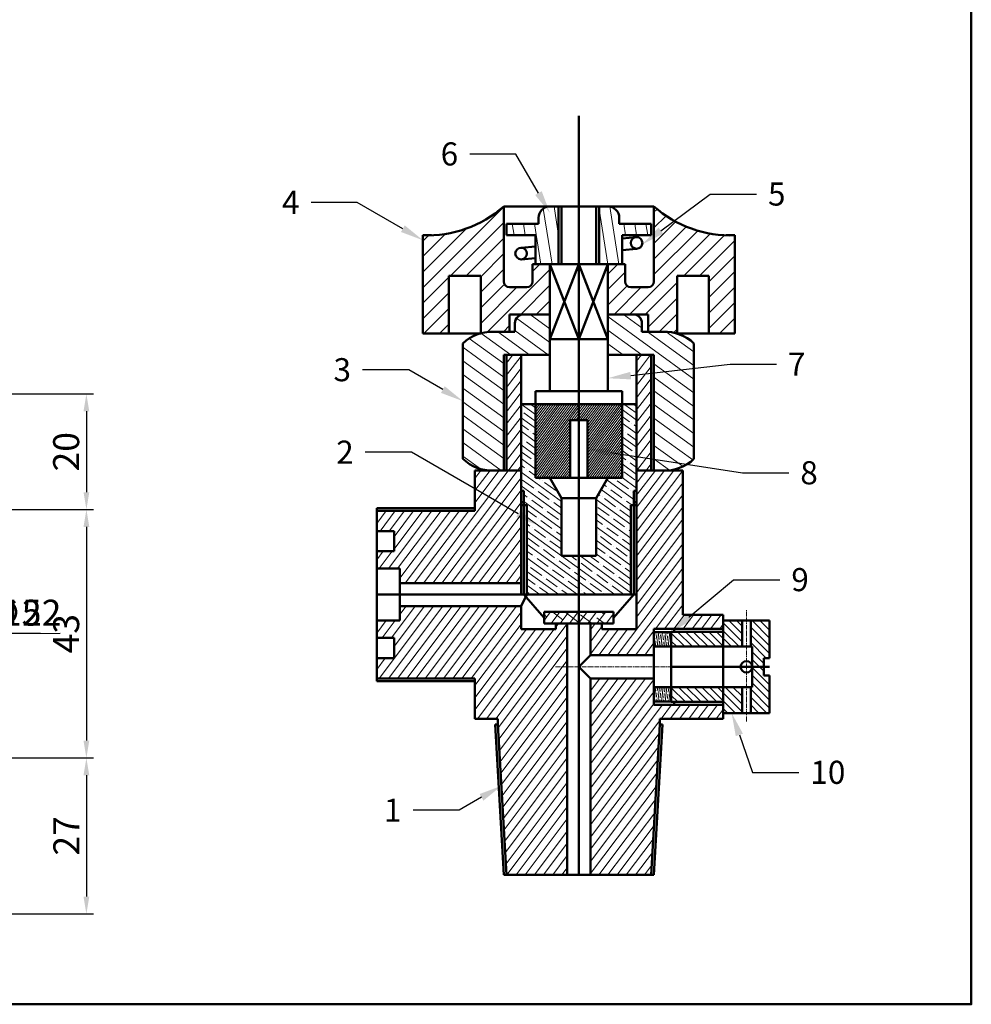
# Model space of a CAD drawing. Units: millimetres. Extents: x 418 to 773, y -46 to 294.
# Tile 6 of 7: x 609 to 773, y -46 to 124. Entities that reach past the tile are written whole.
import ezdxf
from ezdxf import colors
from ezdxf.entities.mleader import LeaderData, LeaderLine
from ezdxf.math import Vec2, Vec3

# ---------------------------------------------------------------- set-up
doc = ezdxf.new("R2010")
doc.units = ezdxf.units.MM
doc.header["$LTSCALE"] = 0.2
doc.linetypes.add('CENTER2', pattern=[28.575, 19.05, -3.175, 3.175, -3.175])
for name, color, linetype, lineweight in [('M-CNTR', 1, 'CENTER2', 18), ('M-DIMS', 2, 'Continuous', 25), ('M-HATC', 8, 'Continuous', 18), ('M-OUTL', 7, 'Continuous', 50), ('M-TEXT', 3, 'Continuous', 25), ('M-TTLB', 7, 'Continuous', 50)]:
    doc.layers.add(name, color=color, linetype=linetype, lineweight=lineweight)
doc.styles.get("Standard").update_dxf_attribs({"font": 'arial.ttf'})
doc.dimstyles.new('ISO-25', dxfattribs={"dimtxt": 4.5, "dimasz": 3, "dimexe": 1.25, "dimexo": 0.625, "dimtad": 1, "dimdec": 1, "dimtxsty": 'Standard', "dimcen": 2.5, "dimadec": 0, "dimazin": 0, "dimtfac": 1, "dimtdec": 1, "dimtmove": 0, "dimatfit": 3, "dimfxl": 1, "dimarcsym": 0})

# ---------------------------------------------------------------- blocks, each defined once
blk = doc.blocks.new('*D90')
at = {"layer": 'Defpoints', "color": 0, "ltscale": 0.2, "transparency": 16777216}
for p in [(600.02, 59.18), (601.02, 39.18), (620.1, 39.18)]:
    blk.add_point(p, dxfattribs=at)
at = {"layer": 'M-DIMS', "color": 0, "lineweight": -2, "ltscale": 0.2, "transparency": 16777216}
for p, q in [((600.64, 59.18), (621.35, 59.18)), ((620.1, 56.18), (620.1, 42.18)), ((601.64, 39.18), (621.35, 39.18))]:
    blk.add_line(p, q, dxfattribs=at)
at = {"layer": 'M-DIMS', "color": 0, "ltscale": 0.2, "transparency": 16777216}
for points in [[(619.6, 56.18), (620.6, 56.18), (620.1, 59.18)], [(619.6, 42.18), (620.6, 42.18), (620.1, 39.18)]]:
    blk.add_solid(points, dxfattribs=at)
at = {"layer": 'M-DIMS', "color": 0, "ltscale": 0.2, "transparency": 16777216, "insert": (617.18, 49.18), "char_height": 4.5, "attachment_point": 5, "rotation": 90}
blk.add_mtext('20', dxfattribs=at)
blk = doc.blocks.new('*D91')
at = {"layer": 'Defpoints', "color": 0, "ltscale": 0.2, "transparency": 16777216}
for p in [(611.5, 39.18), (604.02, -3.82), (620.1, -3.82)]:
    blk.add_point(p, dxfattribs=at)
at = {"layer": 'M-DIMS', "color": 0, "lineweight": -2, "ltscale": 0.2, "transparency": 16777216}
for p, q in [((612.12, 39.18), (621.35, 39.18)), ((620.1, 36.18), (620.1, -0.82)), ((604.64, -3.82), (621.35, -3.82))]:
    blk.add_line(p, q, dxfattribs=at)
at = {"layer": 'M-DIMS', "color": 0, "ltscale": 0.2, "transparency": 16777216}
for points in [[(619.6, 36.18), (620.6, 36.18), (620.1, 39.18)], [(619.6, -0.82), (620.6, -0.82), (620.1, -3.82)]]:
    blk.add_solid(points, dxfattribs=at)
at = {"layer": 'M-DIMS', "color": 0, "ltscale": 0.2, "transparency": 16777216, "insert": (617.18, 17.68), "char_height": 4.5, "attachment_point": 5, "rotation": 90}
blk.add_mtext('43', dxfattribs=at)
blk = doc.blocks.new('*D92')
at = {"layer": 'Defpoints', "color": 0, "ltscale": 0.2, "transparency": 16777216}
for p in [(608.93, -3.82), (592.52, -30.82), (620.1, -30.82)]:
    blk.add_point(p, dxfattribs=at)
at = {"layer": 'M-DIMS', "color": 0, "lineweight": -2, "ltscale": 0.2, "transparency": 16777216}
for p, q in [((609.56, -3.82), (621.35, -3.82)), ((620.1, -6.82), (620.1, -27.82)), ((593.14, -30.82), (621.35, -30.82))]:
    blk.add_line(p, q, dxfattribs=at)
at = {"layer": 'M-DIMS', "color": 0, "ltscale": 0.2, "transparency": 16777216}
for points in [[(619.6, -6.82), (620.6, -6.82), (620.1, -3.82)], [(619.6, -27.82), (620.6, -27.82), (620.1, -30.82)]]:
    blk.add_solid(points, dxfattribs=at)
at = {"layer": 'M-DIMS', "color": 0, "ltscale": 0.2, "transparency": 16777216, "insert": (617.22, -17.32), "char_height": 4.5, "attachment_point": 5, "rotation": 90}
blk.add_mtext('27', dxfattribs=at)
blk = doc.blocks.new('*D102')
at = {"layer": 'Defpoints', "color": 0, "ltscale": 0.2, "transparency": 16777216}
for p in [(575.02, 17.68), (597.02, 17.68)]:
    blk.add_point(p, dxfattribs=at)
at = {"layer": 'M-DIMS', "color": 0, "lineweight": -2, "ltscale": 0.2, "transparency": 16777216}
for p, q in [((572.02, 17.68), (569.02, 17.68)), ((575.02, 17.68), (597.02, 17.68)), ((615.56, 17.69), (600.02, 17.68))]:
    blk.add_line(p, q, dxfattribs=at)
at = {"layer": 'M-DIMS', "color": 0, "ltscale": 0.2, "transparency": 16777216}
for points in [[(572.02, 18.18), (572.02, 17.18), (575.02, 17.68)], [(600.02, 18.19), (600.02, 17.19), (597.02, 17.68)]]:
    blk.add_solid(points, dxfattribs=at)
at = {"layer": 'M-DIMS', "color": 0, "ltscale": 0.2, "transparency": 16777216, "insert": (609.29, 20.73), "char_height": 4.5, "attachment_point": 5, "rotation": 0.0004}
blk.add_mtext('∅22', dxfattribs=at)
blk = doc.blocks.new('*D103')
at = {"layer": 'Defpoints', "color": 0, "ltscale": 0.2, "transparency": 16777216}
for p in [(578.52, 17.68), (593.52, 17.69)]:
    blk.add_point(p, dxfattribs=at)
at = {"layer": 'M-DIMS', "color": 0, "lineweight": -2, "ltscale": 0.2, "transparency": 16777216}
for p, q in [((575.52, 17.68), (572.52, 17.68)), ((578.52, 17.68), (593.52, 17.69)), ((612.14, 17.69), (596.52, 17.69))]:
    blk.add_line(p, q, dxfattribs=at)
at = {"layer": 'M-DIMS', "color": 0, "ltscale": 0.2, "transparency": 16777216}
for points in [[(575.52, 18.18), (575.52, 17.18), (578.52, 17.68)], [(596.52, 18.19), (596.52, 17.19), (593.52, 17.69)]]:
    blk.add_solid(points, dxfattribs=at)
at = {"layer": 'M-DIMS', "color": 0, "ltscale": 0.2, "transparency": 16777216, "insert": (605.83, 20.73), "char_height": 4.5, "attachment_point": 5, "rotation": 0.0006}
blk.add_mtext('∅15', dxfattribs=at)

msp = doc.modelspace()

# ---------------------------------------------------------------- hatches: boundary and pattern name
at = {"layer": 'M-HATC', "ltscale": 0.2}
h = msp.add_hatch(dxfattribs=at)
h.set_pattern_fill('ANSI31', color=256, scale=0.6)
h.paths.add_polyline_path([(732.3444, 86.646, -0.1927282), (718.3444, 91.646), (718.3444, 78.646, -0.41421356), (717.3444, 77.646), (714.3444, 77.646, -0.41421356), (713.3444, 78.646), (713.3444, 81.646), (710.3444, 81.646), (710.3444, 72.9399), (717.3444, 72.9399), (717.3444, 69.9399), (719.8686, 69.9399, -0.08679952), (722.3398, 69.646), (722.3444, 69.646), (722.3444, 79.646), (727.8444, 79.646), (727.8444, 69.646), (732.3444, 69.646)])
h.paths.add_polyline_path([(692.3444, 91.646, -0.1927282), (678.3444, 86.646), (678.3444, 69.646), (682.8444, 69.646), (682.8444, 79.646), (688.3444, 79.646), (688.3444, 69.6846, -0.07535531), (690.4992, 69.9399), (693.3444, 69.9399), (693.3444, 72.9399), (700.3444, 72.9399), (700.3444, 81.646), (697.3444, 81.646), (697.3444, 78.646, -0.41421356), (696.3444, 77.646), (693.3444, 77.646, -0.41421356), (692.3444, 78.646)])
h = msp.add_hatch(dxfattribs=at)
h.set_pattern_fill('ANSI31', color=256, scale=0.6, angle=54)
h.paths.add_polyline_path([(712.8444, 86.646), (717.8444, 86.646), (717.8444, 88.646), (712.3444, 88.646), (712.3444, 89.646, 0.41421356), (710.3444, 91.646), (708.8444, 91.646), (708.8444, 81.646), (712.8444, 81.646)])
h.paths.add_polyline_path([(701.8444, 91.646), (700.3444, 91.646, 0.41421356), (698.3444, 89.646), (698.3444, 88.646), (692.8444, 88.646), (692.8444, 86.646), (697.8444, 86.646), (697.8444, 81.646), (701.8444, 81.646)])
h = msp.add_hatch(dxfattribs=at)
h.set_pattern_fill('ANSI31', color=256, scale=0.6, angle=99)
h.paths.add_polyline_path([(692.3444, 65.9399), (695.3444, 65.9399), (700.3444, 65.9399), (700.3444, 68.646), (700.3444, 72.9399), (695.7641, 72.9399, 0.41421356), (694.2641, 71.4399), (694.2641, 69.9399), (690.029, 69.9399, 0.05904189), (688.3444, 69.6846), (688.3444, 69.646), (688.2094, 69.646, 0.11920158), (685.2641, 67.9399), (685.2641, 47.9399, 0.18451463), (690.029, 45.9399), (692.3444, 45.9399)])
h.paths.add_polyline_path([(725.2641, 67.9399, 0.17937471), (720.6597, 69.9399), (716.2641, 69.9399), (716.2641, 71.4399, 0.41421356), (714.7641, 72.9399), (710.3444, 72.9399), (710.3444, 72.646), (710.3444, 68.646), (710.3444, 65.9399), (715.3444, 65.9399), (718.3444, 65.9399), (718.3444, 45.9399), (720.6597, 45.9399, 0.17937471), (725.2641, 47.9399)])
h = msp.add_hatch(dxfattribs=at)
h.set_pattern_fill('ANSI31', color=256, scale=0.4, angle=8)
h.set_pattern_definition([(53, (-256.1481, -162.8936), (-1.0142671, 0.764305), [])])
h.paths.add_polyline_path([(707.3444, -24.0601), (717.8435, -24.0601), (719.3452, 1.9687), (719.3452, 2.9399), (730.3444, 2.9399), (730.3444, 5.3599), (718.3444, 5.3599), (718.3444, 9.9399), (707.3444, 9.9399)])
h.paths.add_polyline_path([(718.3444, 18.5199), (730.3444, 18.5199), (730.3444, 20.9399), (723.3444, 20.9399), (723.3444, 45.9399), (717.8444, 45.9399), (717.8444, 65.9399), (715.3444, 65.9399), (715.3444, 39.9399), (715.3444, 24.4399), (715.3444, 18.4399), (709.3444, 18.4399), (709.3444, 19.4399), (707.3444, 19.4399), (707.3444, 13.9399), (718.3444, 13.9399)])
h.paths.add_polyline_path([(695.3444, 39.9399), (695.3444, 65.9399), (692.8444, 65.9399), (692.8444, 45.9399), (687.3444, 45.9399), (687.3444, 38.9399), (670.3444, 38.9399), (670.3444, 35.4399), (673.3444, 35.4399), (673.3444, 31.9399), (670.3444, 31.9399), (670.3444, 28.9399), (674.3444, 28.9399), (674.3444, 26.4399), (695.3444, 26.4399)])
h.paths.add_polyline_path([(687.3444, 9.9399), (687.3444, 2.9399), (691.3444, 2.9399), (691.3444, 1.9543), (692.8452, -24.0601), (703.3444, -24.0601), (703.3444, 19.4399), (701.3444, 19.4399), (701.3444, 18.4399), (695.3444, 18.4399), (695.3444, 22.4399), (674.3444, 22.4399), (674.3444, 19.9399), (670.3444, 19.9399), (670.3444, 16.9399), (673.3444, 16.9399), (673.3444, 13.4399), (670.3444, 13.4399), (670.3444, 9.9399)])
h = msp.add_hatch(dxfattribs=at)
h.set_pattern_fill('ANSI35', color=256, scale=0.3, angle=99)
h.set_pattern_definition([(144, (565.0857, -356.5551), (-1.119731, -1.541177), []), (144, (564.875, -355.2247), (-1.119731, -1.541177), [2.38125, -0.47625, 0, -0.47625])])
h.paths.add_polyline_path([(714.3444, 39.9399), (714.8444, 39.9399), (714.8444, 40.4399), (714.8444, 42.4399), (715.3444, 42.4399), (715.3444, 57.4399), (712.8444, 57.4399), (712.8444, 44.646), (710.3651, 44.646), (708.3444, 41.146), (708.3444, 31.146), (705.3444, 31.146), (705.3444, 24.4399), (714.3444, 24.4399)])
h.paths.add_polyline_path([(702.3444, 41.146), (700.3236, 44.646), (697.8444, 44.646), (697.8444, 57.4399), (695.3444, 57.4399), (695.3444, 42.4399), (695.8444, 42.4399), (695.8444, 40.4399), (695.8444, 39.9399), (696.3444, 39.9399), (696.3444, 24.4399), (705.3444, 24.4399), (705.3444, 31.146), (702.3444, 31.146)])
h = msp.add_hatch(dxfattribs=at)
h.set_pattern_fill('ANSI31', color=256, scale=0.1, angle=8)
h.set_pattern_definition([(53, (565.08574, -356.55513), (-0.25356677, 0.19107627), [])])
h.paths.add_polyline_path([(712.8444, 57.4399), (705.3444, 57.4399), (705.3444, 54.646), (706.8444, 54.646), (706.8444, 45.9399), (712.8444, 45.9399)])
h.paths.add_polyline_path([(703.8444, 54.646), (705.3444, 54.646), (705.3444, 57.4399), (697.8444, 57.4399), (697.8444, 45.9399), (703.8444, 45.9399)])
h.paths.add_polyline_path([(703.8444, 45.9399), (697.8444, 45.9399), (697.8444, 44.646), (703.8444, 44.646)])
h.paths.add_polyline_path([(712.8444, 45.9399), (706.8444, 45.9399), (706.8444, 44.646), (712.8444, 44.646)])
h = msp.add_hatch(dxfattribs=at)
h.set_pattern_fill('ANSI38', color=256, scale=0.4, angle=8)
h.set_pattern_definition([(53, (565.0857, -356.5551), (-1.014267, 0.764305), []), (143, (565.0857, -356.5551), (-2.7928393, 0.514343), [3.175, -1.905])])
h.paths.add_polyline_path([(711.3444, 20.4399), (711.3444, 21.4399), (705.3444, 21.4399), (705.3444, 19.4399), (711.3444, 19.4399)])
h.paths.add_polyline_path([(705.3444, 21.4399), (699.3444, 21.4399), (699.3444, 20.4399), (699.3444, 19.4399), (705.3444, 19.4399)])
h = msp.add_hatch(dxfattribs=at)
h.set_pattern_fill('ANSI31', color=256, scale=0.3, angle=90)
h.set_pattern_definition([(135, (146.1118, -196.371), (-0.6735192, -0.6735192), [])])
h.paths.add_polyline_path([(733.5944, 19.9399), (730.3444, 19.9399), (730.3444, 18.0199), (721.3444, 18.0199), (721.3444, 15.4399), (733.5944, 15.4399)])
h.paths.add_polyline_path([(738.3444, 19.9399), (735.0944, 19.9399), (735.0944, 15.4399), (735.3444, 15.4399), (735.3444, 11.9399), (737.3444, 11.9399), (737.3444, 13.4399), (738.3444, 13.4399)])
h.paths.add_polyline_path([(733.5944, 8.4399), (721.3444, 8.4399), (721.3444, 5.8599), (730.3444, 5.8599), (730.3444, 3.9399), (733.5944, 3.9399)])
h.paths.add_polyline_path([(738.3444, 10.4399), (737.3444, 10.4399), (737.3444, 11.9399), (735.3444, 11.9399), (735.3444, 8.4399), (735.0944, 8.4399), (735.0944, 3.9399), (738.3444, 3.9399)])
h = msp.add_hatch(dxfattribs=at)
h.set_pattern_fill('ANSI35', color=256, scale=0.1, angle=38)
h.set_pattern_definition([(83, (565.08574, -356.5551), (-0.6302668, 0.077387), []), (83, (565.43957, -356.2787), (-0.6302668, 0.077387), [0.79375, -0.15875, 0, -0.15875])])
h.paths.add_polyline_path([(718.3444, 17.9399), (718.3444, 15.4399), (721.3444, 15.4399), (721.3444, 17.9399)])
h.paths.add_polyline_path([(718.3444, 8.4399), (718.3444, 5.9399), (721.3444, 5.9399), (721.3444, 8.4399)])

# ---------------------------------------------------------------- linework, layer by layer
at = {"layer": 'M-CNTR', "ltscale": 0.2}
for p, q in [((734.3444, 2.4763), (734.3444, 21.823)), ((731.7399, 11.9399), (701.3091, 11.9399))]:
    msp.add_line(p, q, dxfattribs=at)
at = {"layer": 'M-OUTL', "ltscale": 0.2}
for p, q in [((705.3444, 107.3265), (705.3444, 19.4399)), ((718.3444, 91.646), (692.3444, 91.646)), ((692.3444, 91.646), (692.3444, 78.646)), ((710.3444, 91.646), (700.3444, 91.646)), ((701.8444, 91.646), (701.8444, 81.646)), ((702.3444, 91.646), (702.3444, 81.646)), ((705.3444, 91.646), (705.3444, 81.646)), ((708.3444, 91.646), (708.3444, 81.646)), ((708.8444, 91.646), (708.8444, 81.646)), ((718.3444, 91.646), (718.3444, 78.646)), ((692.8444, 88.646), (692.8444, 86.6989)), ((698.3444, 88.646), (692.8444, 88.646)), ((698.3444, 89.646), (698.3444, 88.646)), ((712.3444, 88.646), (712.3444, 89.646)), ((717.8444, 88.646), (712.3444, 88.646)), ((717.8444, 88.646), (717.8444, 86.646)), ((678.3444, 86.646), (678.3444, 69.646)), ((679.8545, 86.646), (678.3444, 86.646)), ((692.8444, 86.6989), (692.8444, 86.646)), ((692.8444, 86.646), (697.8444, 86.646)), ((697.8444, 86.646), (697.8444, 81.646)), ((712.8444, 81.646), (712.8444, 86.646)), ((712.8444, 86.646), (717.8444, 86.646)), ((712.8444, 86.0925), (715.2533, 86.3127)), ((732.3444, 86.646), (730.8342, 86.646)), ((732.3444, 69.646), (732.3444, 86.646)), ((695.3444, 84.4928), (697.8444, 84.7213)), ((705.3444, 81.646), (705.3444, 85.1553)), ((712.8444, 84.0878), (715.3444, 84.3168)), ((695.3444, 82.4845), (697.8444, 82.7135)), ((713.3444, 81.646), (697.3444, 81.646)), ((697.3444, 78.646), (697.3444, 81.646)), ((697.8444, 81.646), (705.3444, 81.646)), ((700.3444, 72.646), (700.3444, 81.646)), ((705.3444, 81.646), (712.8444, 81.646)), ((710.3444, 72.646), (710.3444, 81.646)), ((713.3444, 78.646), (713.3444, 81.646)), ((682.8444, 69.646), (682.8444, 79.646)), ((682.8444, 79.646), (688.3444, 79.646)), ((688.3444, 69.646), (688.3444, 79.646)), ((722.3444, 69.646), (722.3444, 79.646)), ((727.8444, 79.646), (722.3444, 79.646)), ((727.8444, 69.646), (727.8444, 79.646)), ((693.3444, 77.646), (696.3444, 77.646)), ((717.3444, 77.646), (714.3444, 77.646)), ((693.3444, 72.9399), (693.3444, 69.9399)), ((700.3444, 72.9399), (693.3444, 72.9399)), ((700.3444, 72.9399), (695.7641, 72.9399)), ((714.7641, 72.9399), (710.3444, 72.9399)), ((714.7641, 72.9399), (710.3444, 72.9399)), ((710.3444, 72.9399), (714.7641, 72.9399)), ((717.3444, 72.9399), (710.3444, 72.9399)), ((717.3444, 69.9399), (717.3444, 72.9399)), ((694.2641, 69.9399), (690.029, 69.9399)), ((694.2641, 71.4399), (694.2641, 69.9399)), ((694.2641, 71.4399), (694.2641, 69.9399)), ((716.2641, 69.9399), (716.2641, 71.4399)), ((720.6597, 69.9399), (716.2641, 69.9399)), ((678.3444, 69.646), (688.3444, 69.646)), ((722.3398, 69.646), (732.3444, 69.646)), ((685.2641, 67.9399), (685.2641, 47.9399)), ((725.2641, 47.9399), (725.2641, 67.9399)), ((695.3444, 65.9399), (692.3444, 65.9399)), ((692.3444, 65.9399), (692.3444, 45.9399)), ((692.8444, 65.9399), (692.8444, 45.9399)), ((695.3444, 65.9399), (700.3444, 65.9399)), ((695.3444, 39.9399), (695.3444, 65.9399)), ((710.3444, 65.9399), (715.3444, 65.9399)), ((715.3444, 65.9399), (715.3444, 39.9399)), ((715.3444, 65.9399), (718.3444, 65.9399)), ((717.8444, 65.9399), (717.8444, 45.9399)), ((718.3444, 65.9399), (718.3444, 45.9399)), ((695.3444, 57.4399), (715.3444, 57.4399)), ((695.3444, 57.4399), (695.3444, 42.4399)), ((705.3444, 57.4399), (705.3444, 19.4399)), ((715.3444, 42.4399), (715.3444, 57.4399)), ((692.8444, 45.9399), (687.3444, 45.9399)), ((687.3444, 45.9399), (687.3444, 39.4399)), ((687.3444, 38.9399), (687.3444, 45.9399)), ((690.029, 45.9399), (695.3444, 45.9399)), ((692.8444, 45.9399), (695.3444, 45.9399)), ((702.3444, 41.146), (700.3236, 44.646)), ((700.3236, 44.646), (706.8444, 44.646)), ((708.3444, 41.146), (710.3651, 44.646)), ((715.3444, 45.9399), (717.8444, 45.9399)), ((715.3444, 45.9399), (720.6597, 45.9399)), ((717.8444, 45.9399), (723.3444, 45.9399)), ((723.3444, 45.9399), (723.3444, 20.9399)), ((695.8444, 42.4399), (695.3444, 42.4399)), ((695.8444, 42.4399), (695.8444, 40.4399)), ((702.3444, 31.146), (702.3444, 41.146)), ((702.3444, 41.146), (705.3444, 41.146)), ((705.3444, 41.146), (708.3444, 41.146)), ((708.3444, 41.146), (708.3444, 31.146)), ((714.8444, 42.4399), (715.3444, 42.4399)), ((714.8444, 42.4399), (714.8444, 40.4399)), ((670.3444, 24.4399), (670.3444, 39.4399)), ((670.3444, 24.4399), (670.3444, 39.4399)), ((670.3444, 39.4399), (687.3444, 39.4399)), ((695.3444, 40.4399), (695.8444, 40.4399)), ((695.3444, 40.4399), (695.3444, 24.4399)), ((695.3444, 39.9399), (695.3444, 26.4399)), ((696.3444, 39.9399), (695.3444, 39.9399)), ((695.8444, 40.4399), (695.8444, 24.4399)), ((696.3444, 24.4399), (696.3444, 39.9399)), ((715.3444, 39.9399), (714.3444, 39.9399)), ((714.3444, 39.9399), (714.3444, 24.4399)), ((714.8444, 40.4399), (714.8444, 24.4399)), ((714.8444, 40.4399), (715.3444, 40.4399)), ((715.3444, 24.4399), (715.3444, 40.4399)), ((715.3444, 39.9399), (715.3444, 24.4399)), ((670.3444, 38.9399), (687.3444, 38.9399)), ((670.3444, 35.4399), (673.3444, 35.4399)), ((673.3444, 35.4399), (673.3444, 31.9399)), ((673.3444, 31.9399), (670.3444, 31.9399)), ((708.3444, 31.146), (702.3444, 31.146)), ((670.3444, 28.9399), (674.3444, 28.9399)), ((674.3444, 28.9399), (674.3444, 19.9399)), ((674.3444, 26.4399), (695.3444, 26.4399)), ((670.3444, 24.4399), (715.3444, 24.4399)), ((670.3444, 24.4399), (670.3444, 9.4399)), ((695.3444, 24.4399), (705.3444, 24.4399)), ((695.3444, 22.4399), (696.3444, 24.4399)), ((699.3444, 20.4399), (695.8444, 24.4399)), ((711.3444, 20.4399), (714.8444, 24.4399)), ((714.8444, 24.4399), (715.3444, 24.4399)), ((715.3444, 24.4399), (715.3444, 18.4399)), ((674.3444, 22.4399), (695.3444, 22.4399)), ((695.3444, 22.4399), (695.3444, 18.4399)), ((705.3444, 21.4399), (699.3444, 21.4399)), ((699.3444, 21.4399), (699.3444, 21.4399)), ((699.3444, 21.4399), (699.3444, 20.4399)), ((711.3444, 21.4399), (705.3444, 21.4399)), ((711.3444, 20.4399), (711.3444, 21.4399)), ((730.3444, 20.9399), (723.3444, 20.9399)), ((730.3444, 11.9399), (730.3444, 20.9399)), ((674.3444, 19.9399), (670.3444, 19.9399)), ((699.3444, 20.4399), (699.3444, 19.4399)), ((699.3444, 19.4399), (711.3444, 19.4399)), ((701.3444, 19.4399), (705.3444, 19.4399)), ((701.3444, 19.4399), (701.3444, 18.4399)), ((703.3444, 19.4399), (703.3444, -24.0601)), ((705.3444, 19.4399), (705.3444, -24.0601)), ((709.3444, 19.4399), (705.3444, 19.4399)), ((707.3444, 19.4399), (707.3444, 13.9399)), ((709.3444, 18.4399), (709.3444, 19.4399)), ((711.3444, 19.4399), (711.3444, 20.4399)), ((730.3444, 18.0199), (730.3444, 19.9399)), ((730.3444, 19.9399), (738.3444, 19.9399)), ((733.5944, 15.4399), (733.5944, 19.9399)), ((735.0944, 15.4399), (735.0944, 19.9399)), ((738.3444, 19.9399), (738.3444, 13.4399)), ((695.3444, 18.4399), (701.3444, 18.4399)), ((715.3444, 18.4399), (709.3444, 18.4399)), ((730.3444, 18.5199), (718.3444, 18.5199)), ((718.3444, 18.5199), (718.3444, 5.3599)), ((721.3444, 5.8599), (721.3444, 18.0199)), ((721.3444, 18.0199), (730.3444, 18.0199)), ((721.8444, 18.5199), (730.3444, 18.5199)), ((721.8444, 18.0199), (721.8444, 18.5199)), ((673.3444, 16.9399), (670.3444, 16.9399)), ((673.3444, 13.4399), (673.3444, 16.9399)), ((721.3444, 15.4399), (735.3444, 15.4399)), ((735.3444, 15.4399), (735.3444, 8.4399)), ((705.3444, 11.9399), (707.3444, 13.9399)), ((718.3444, 13.9399), (707.3444, 13.9399)), ((670.3444, 13.4399), (673.3444, 13.4399)), ((705.3444, 11.9399), (707.3444, 9.9399)), ((721.3444, 11.9399), (738.3444, 11.9399)), ((730.3444, 11.9399), (730.3444, 2.9399)), ((738.3444, 13.4399), (737.3444, 13.4399)), ((737.3444, 13.4399), (737.3444, 10.4399)), ((737.3444, 10.4399), (738.3444, 10.4399)), ((738.3444, 10.4399), (738.3444, 3.9399)), ((670.3444, 9.9399), (687.3444, 9.9399)), ((670.3444, 9.4399), (687.3444, 9.4399)), ((687.3444, 9.9399), (687.3444, 2.9399)), ((707.3444, 9.9399), (707.3444, -24.0601)), ((718.3444, 9.9399), (707.3444, 9.9399)), ((735.3444, 8.4399), (721.3444, 8.4399)), ((733.5944, 3.9399), (733.5944, 8.4399)), ((735.0944, 3.9399), (735.0944, 8.4399)), ((718.3444, 5.3599), (730.3444, 5.3599)), ((721.3444, 5.8599), (730.3444, 5.8599)), ((721.8444, 5.8599), (721.8444, 5.3599)), ((721.8444, 5.3599), (730.3444, 5.3599)), ((730.3444, 3.9399), (730.3444, 5.8599)), ((738.3444, 3.9399), (730.3444, 3.9399)), ((691.3444, 2.9399), (687.3444, 2.9399)), ((690.8444, 1.9399), (691.3452, 1.9399)), ((690.8444, 1.9399), (692.3444, -24.0601)), ((691.3435, 1.9687), (692.8435, -24.0313)), ((691.3444, 1.9399), (691.3444, 2.9399)), ((705.3444, 2.9399), (705.3444, 1.9399)), ((719.3452, 1.9687), (717.8452, -24.0313)), ((718.3444, -24.0601), (719.8444, 1.9399)), ((719.3435, 1.9399), (719.8444, 1.9399)), ((730.3444, 2.9399), (719.3452, 2.9399)), ((719.3452, 1.9687), (719.3452, 2.9399)), ((692.3444, -24.0601), (718.3444, -24.0601)), ((705.3444, -24.0601), (703.3444, -24.0601)), ((705.3444, -24.0601), (718.3444, -24.0601))]:
    msp.add_line(p, q, dxfattribs=at)
at = {"layer": 'M-OUTL'}
for p, q in [((700.3444, 68.646), (700.3444, 81.646)), ((700.3444, 81.646), (701.8444, 81.646)), ((700.3444, 81.646), (705.3444, 68.646)), ((700.3444, 68.646), (705.3444, 81.646)), ((701.8444, 81.646), (708.8444, 81.646)), ((705.3444, 81.646), (710.3444, 81.646)), ((705.3444, 68.646), (710.3444, 81.646)), ((705.3444, 81.646), (710.3444, 68.646)), ((710.3444, 81.646), (710.3444, 68.646)), ((710.3444, 68.646), (700.3444, 68.646)), ((700.3444, 68.646), (700.3444, 59.646)), ((710.3444, 68.646), (710.3444, 59.646)), ((712.8444, 59.646), (697.8444, 59.646)), ((697.8444, 59.646), (697.8444, 44.646)), ((712.8444, 44.646), (712.8444, 59.646)), ((703.8444, 44.646), (703.8444, 54.646)), ((703.8444, 54.646), (706.8444, 54.646)), ((706.8444, 54.646), (706.8444, 44.646)), ((697.8444, 44.646), (703.8444, 44.646)), ((706.8444, 44.646), (712.8444, 44.646))]:
    msp.add_line(p, q, dxfattribs=at)
at = {"layer": 'M-OUTL', "ltscale": 0.5}
for p, q in [((718.3444, 17.9399), (718.3444, 5.9399)), ((721.3444, 17.9399), (718.3444, 17.9399)), ((721.3444, 5.9399), (721.3444, 17.9399)), ((718.3444, 15.4399), (721.3444, 15.4399)), ((718.3444, 8.4399), (721.3444, 8.4399)), ((718.3444, 5.9399), (721.3444, 5.9399))]:
    msp.add_line(p, q, dxfattribs=at)
at = {"layer": 'M-OUTL', "ltscale": 0.2}
for centre, radius in [((715.3444, 85.3168), 1), ((695.3444, 83.4887), 1.0042), ((734.3444, 11.9399), 1)]:
    msp.add_circle(centre, radius, dxfattribs=at)
for centre, radius, start, end in [((679.0994, 106.6318), 20, 267.836305, 311.471343), ((700.3444, 89.646), 2, 90, 180), ((710.3444, 89.646), 2, 0, 90), ((731.5893, 106.6318), 20, 228.528657, 272.163695), ((693.3444, 78.646), 1, 180, 270), ((696.3444, 78.646), 1, 270, 0), ((714.3444, 78.646), 1, 180, 270), ((717.3444, 78.646), 1, 270, 0), ((695.7641, 71.4399), 1.5, 90, 180), ((714.7641, 71.4399), 1.5, 0, 90), ((690.2641, 62.7037), 7.24, 88.139064, 133.678241), ((720.2641, 62.729), 7.2217, 46.183162, 93.139767), ((690.2641, 53.1761), 7.24, 226.321759, 271.860936), ((720.2641, 53.1508), 7.2217, 266.860233, 313.816838)]:
    msp.add_arc(centre, radius, start, end, dxfattribs=at)
at = {"layer": 'M-TTLB', "ltscale": 0.2}
msp.add_lwpolyline([(417.9371, 294.4119), (773.2687, 294.4119), (773.2687, -46.4726), (417.9371, -46.4726)], close=True, dxfattribs=at)

# ---------------------------------------------------------------- dimensions: what is measured, and where the dimension line sits
at = {"layer": 'M-DIMS', "ltscale": 0.2}
for base, p1, p2, picture, middle in [((620.1049, 39.1849), (600.0171, 59.1849), (601.0171, 39.1849), '*D90', (617.1824, 49.1849)), ((620.1049, -3.8151), (611.4985, 39.1849), (604.0171, -3.8151), '*D91', (617.1808, 17.6849)), ((620.1049, -30.8151), (608.9306, -3.8151), (592.5171, -30.8151), '*D92', (617.2207, -17.3151))]:
    dim = msp.add_linear_dim(base=base, p1=p1, p2=p2, angle=90, dimstyle='ISO-25', override={"dimclrd": 0, "dimclre": 0, "dimclrt": 0}, dxfattribs=at)
    dim.commit()
    dim.dimension.update_dxf_attribs({"geometry": picture, "text_midpoint": middle})
for p1, p2, picture, middle in [((575.0171, 17.6848), (597.0171, 17.685), '*D102', (609.2902, 17.6851)), ((578.5171, 17.6848), (593.5171, 17.685), '*D103', (605.8301, 17.6851))]:
    dim = msp.add_diameter_dim_2p(p1=p1, p2=p2, dimstyle='ISO-25', override={"dimdec": 0, "dimlfac": 1, "dimrnd": 0, "dimzin": 0, "dimdsep": 46, "dimlunit": 2}, dxfattribs=at)
    dim.commit()
    dim.dimension.update_dxf_attribs({"geometry": picture, "text_midpoint": middle})

# ---------------------------------------------------------------- leaders
at = {"layer": 'M-TEXT', "ltscale": 0.2}
ml = msp.add_multileader_mtext('Standard', dxfattribs=at)
ml.set_content('6', color=256)
ml.set_leader_properties()
ml.build(insert=Vec2(0, 0))
ctx = ml.context
ctx.base_point, ctx.plane_origin = Vec3(679.8108, 100.6972), Vec3(700.3444, 90.4913)
ctx.text_align_type = 2
notes = []
notes.append((ctx, [(0, (1, 1, 0), (694.452, 100.6972), (-1, 0), 8, [(0, [(700.3444, 90.4913)], 0, [])])]))
ctx.mtext.insert, ctx.mtext.alignment, ctx.mtext.flow_direction = Vec3(684.452, 102.7314), 3, 5
ml = msp.add_multileader_mtext('Standard', dxfattribs=at)
ml.set_content('5', color=256)
ml.set_leader_properties()
ml.build(insert=Vec2(0, 0))
ctx = ml.context
ctx.base_point, ctx.plane_origin = Vec3(736.0794, 93.7595), Vec3(716.3139, 85.0719)
notes.append((ctx, [(0, (1, 1, 0), (728.0794, 93.7595), (1, 0), 8, [(0, [(716.3139, 85.0719)], 0, [])])]))
ctx.mtext.insert, ctx.mtext.flow_direction = Vec3(738.0794, 95.7936), 5
ml = msp.add_multileader_mtext('Standard', dxfattribs=at)
ml.set_content('4', color=256)
ml.set_leader_properties()
ml.build(insert=Vec2(0, 0))
ctx = ml.context
ctx.base_point, ctx.plane_origin = Vec3(652.2171, 92.3505), Vec3(678.3444, 85.7915)
ctx.text_align_type = 2
notes.append((ctx, [(0, (1, 1, 0), (666.9838, 92.3505), (-1, 0), 8, [(0, [(678.3444, 85.7915)], 0, [])])]))
ctx.mtext.insert, ctx.mtext.alignment, ctx.mtext.flow_direction = Vec3(656.9838, 94.3505), 3, 5
ml = msp.add_multileader_mtext('Standard', dxfattribs=at)
ml.set_content('3', color=256)
ml.set_leader_properties()
ml.build(insert=Vec2(0, 0))
ctx = ml.context
ctx.base_point, ctx.plane_origin = Vec3(661.2822, 63.3454), Vec3(685.2641, 57.9399)
ctx.text_align_type = 2
notes.append((ctx, [(0, (1, 1, 0), (675.9016, 63.3454), (-1, 0), 8, [(0, [(685.2641, 57.9399)], 0, [])])]))
ctx.mtext.insert, ctx.mtext.alignment, ctx.mtext.flow_direction = Vec3(665.9016, 65.3809), 3, 5
ml = msp.add_multileader_mtext('Standard', dxfattribs=at)
ml.set_content('7', color=256)
ml.set_leader_properties()
ml.build(insert=Vec2(0, 0))
ctx = ml.context
ctx.base_point, ctx.plane_origin = Vec3(739.5281, 64.3234), Vec3(710.3444, 61.9016)
notes.append((ctx, [(0, (1, 1, 0), (731.5281, 64.3234), (1, 0), 8, [(0, [(710.3444, 61.9016)], 0, [])])]))
ctx.mtext.insert, ctx.mtext.flow_direction = Vec3(741.5281, 66.3234), 5
ml = msp.add_multileader_mtext('Standard', dxfattribs=at)
ml.set_content('2', color=256)
ml.set_leader_properties()
ml.build(insert=Vec2(0, 0))
ctx = ml.context
ctx.base_point, ctx.plane_origin = Vec3(661.7134, 49.1056), Vec3(698.2978, 36.4415)
ctx.text_align_type = 2
notes.append((ctx, [(0, (1, 1, 0), (676.3628, 49.1056), (-1, 0), 8, [(0, [(698.2978, 36.4415)], 0, [])])]))
ctx.mtext.insert, ctx.mtext.alignment, ctx.mtext.flow_direction = Vec3(666.3628, 51.1056), 3, 5
ml = msp.add_multileader_mtext('Standard', dxfattribs=at)
ml.set_content('8', color=256)
ml.set_leader_properties()
ml.build(insert=Vec2(0, 0))
ctx = ml.context
ctx.base_point, ctx.plane_origin = Vec3(741.6717, 45.5039), Vec3(706.8444, 49.646)
notes.append((ctx, [(0, (1, 1, 0), (733.6717, 45.5039), (1, 0), 8, [(0, [(706.8444, 49.646)], 0, [])])]))
ctx.mtext.insert, ctx.mtext.flow_direction = Vec3(743.6717, 47.538), 5
ml = msp.add_multileader_mtext('Standard', dxfattribs=at)
ml.set_content('9', color=256)
ml.set_leader_properties()
ml.build(insert=Vec2(0, 0))
ctx = ml.context
ctx.base_point, ctx.plane_origin = Vec3(740.1134, 27.0088), Vec3(721.3444, 17.9399)
notes.append((ctx, [(0, (1, 1, 0), (732.1134, 27.0088), (1, 0), 8, [(0, [(721.3444, 17.9399)], 0, [])])]))
ctx.mtext.insert, ctx.mtext.flow_direction = Vec3(742.1134, 29.0429), 5
ml = msp.add_multileader_mtext('Standard', dxfattribs=at)
ml.set_content('10', color=256)
ml.set_leader_properties()
ml.build(insert=Vec2(0, 0))
ctx = ml.context
ctx.base_point, ctx.plane_origin = Vec3(743.4145, -6.3472), Vec3(731.7876, 3.9399)
notes.append((ctx, [(0, (1, 1, 0), (735.4145, -6.3472), (1, 0), 8, [(0, [(731.7876, 3.9399)], 0, [])])]))
ctx.mtext.insert, ctx.mtext.flow_direction = Vec3(745.4145, -4.3131), 5
ml = msp.add_multileader_mtext('Standard', dxfattribs=at)
ml.set_content('1', color=256)
ml.set_leader_properties()
ml.build(insert=Vec2(0, 0))
ctx = ml.context
ctx.base_point, ctx.plane_origin = Vec3(671.1585, -12.8703), Vec3(691.9557, -8.6419)
ctx.text_align_type = 2
notes.append((ctx, [(0, (1, 1, 0), (684.6319, -12.8703), (-1, 0), 8, [(0, [(691.9557, -8.6419)], 0, [])])]))
ctx.mtext.insert, ctx.mtext.alignment, ctx.mtext.flow_direction = Vec3(674.6319, -10.8703), 3, 5
for ctx, leaders in notes:
    for number, flags, end, landing, length, lines in leaders:
        leader = LeaderData()
        leader.index, (leader.has_last_leader_line, leader.has_dogleg_vector, leader.attachment_direction) = number, flags
        leader.last_leader_point, leader.dogleg_vector, leader.dogleg_length = Vec3(end), Vec3(landing), length
        for number, points, colour, breaks in lines:
            line = LeaderLine()
            line.index, line.vertices, line.color, line.breaks = number, Vec3.list(points), colors.encode_raw_color(colour), breaks
            leader.lines.append(line)
        ctx.leaders.append(leader)

doc.saveas('drawing.dxf')
